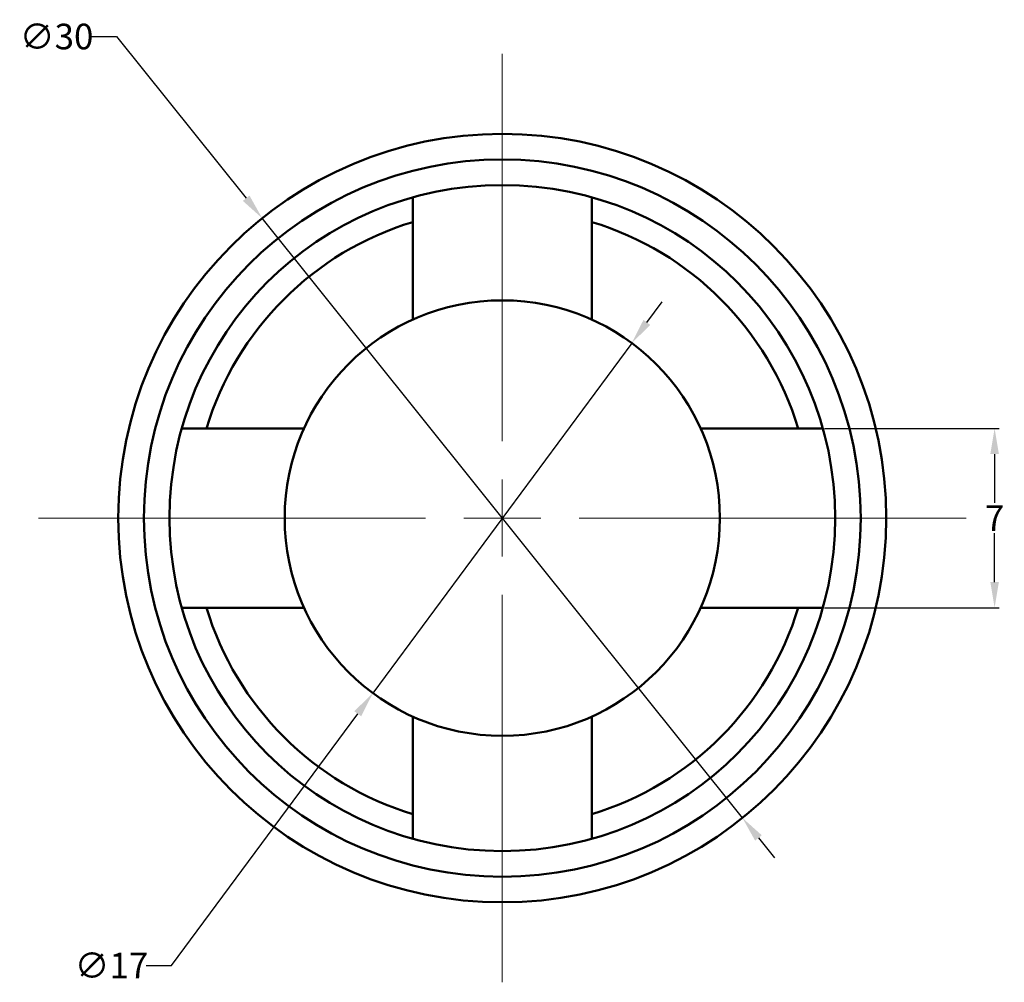
# Model space of a CAD drawing. Units: millimetres. Extents: x 31 to 232, y 35 to 192.
# Tile 4 of 5: x 43 to 82, y 154 to 192. Entities that reach past the tile are written whole.
import ezdxf

# ---------------------------------------------------------------- set-up
doc = ezdxf.new("R2010")
doc.units = ezdxf.units.MM
doc.header["$MEASUREMENT"] = 0
doc.linetypes.add('CENTER', pattern=[50.8, 31.75, -6.35, 6.35, -6.35])
for name, color, linetype, lineweight in [('M-CNTR', 1, 'CENTER', 18), ('M-DIMS', 2, 'Continuous', 25), ('M-OUTL', 7, 'Continuous', 50)]:
    doc.layers.add(name, color=color, linetype=linetype, lineweight=lineweight)
doc.styles.get("Standard").update_dxf_attribs({"font": 'arial.ttf'})
doc.dimstyles.get("Standard").update_dxf_attribs({"dimtxt": 1, "dimasz": 1, "dimexe": 0.18, "dimexo": 0.0625, "dimgap": 0.09, "dimtad": 0, "dimtih": 1, "dimtoh": 1, "dimdec": 0, "dimzin": 0, "dimdsep": 46, "dimtxsty": 'Standard', "dimcen": 0.09, "dimadec": 0, "dimazin": 0, "dimtfac": 1, "dimtdec": 0, "dimtofl": 0, "dimtmove": 0, "dimatfit": 3, "dimfxl": 1, "dimtolj": 1, "dimtzin": 0, "dimarcsym": 0})

# ---------------------------------------------------------------- blocks, each defined once
blk = doc.blocks.new('*U32')
at = {"layer": 'M-CNTR', "color": 0, "transparency": 16777216}
for p, q in [((0, 3), (0, 18.12)), ((-18.12, 0), (-3, 0)), ((3, 0), (18.12, 0)), ((0, -18.12), (0, -3))]:
    blk.add_line(p, q, dxfattribs=at)
at = {"layer": 'M-CNTR', "color": 0, "linetype": 'Continuous', "transparency": 16777216}
for p, q in [((0, -1.5), (0, 1.5)), ((-1.5, 0), (1.5, 0))]:
    blk.add_line(p, q, dxfattribs=at)
blk = doc.blocks.new('*D39')
at = {"layer": 'Defpoints', "color": 0, "transparency": 16777216}
for p in [(74.596, 175.753), (74.596, 168.753), (81.307, 168.753)]:
    blk.add_point(p, dxfattribs=at)
at = {"layer": 'M-DIMS', "color": 0, "lineweight": -2, "transparency": 16777216}
for p, q in [((74.659, 175.753), (81.487, 175.753)), ((81.307, 174.753), (81.307, 172.843)), ((81.307, 169.753), (81.307, 171.663)), ((74.659, 168.753), (81.487, 168.753))]:
    blk.add_line(p, q, dxfattribs=at)
at = {"layer": 'M-DIMS', "color": 0, "transparency": 16777216}
for points in [[(81.14, 174.753), (81.474, 174.753), (81.307, 175.753)], [(81.14, 169.753), (81.474, 169.753), (81.307, 168.753)]]:
    blk.add_solid(points, dxfattribs=at)
at = {"layer": 'M-DIMS', "color": 0, "transparency": 16777216, "insert": (81.307, 172.253), "char_height": 1, "attachment_point": 5}
blk.add_mtext('\\A1;7', dxfattribs=at)
blk = doc.blocks.new('*D40')
at = {"layer": 'Defpoints', "color": 0, "transparency": 16777216}
for p in [(52.696, 183.959), (71.456, 160.548)]:
    blk.add_point(p, dxfattribs=at)
at = {"layer": 'M-DIMS', "color": 0, "lineweight": -2, "transparency": 16777216}
for p, q in [((46.011, 191.053), (47.011, 191.053)), ((47.011, 191.053), (52.071, 184.739)), ((71.456, 160.548), (52.696, 183.959)), ((72.081, 159.767), (72.707, 158.987))]:
    blk.add_line(p, q, dxfattribs=at)
at = {"layer": 'M-DIMS', "color": 0, "transparency": 16777216}
for points in [[(52.201, 184.843), (51.941, 184.635), (52.696, 183.959)], [(72.211, 159.872), (71.951, 159.663), (71.456, 160.548)]]:
    blk.add_solid(points, dxfattribs=at)
at = {"layer": 'M-DIMS', "color": 0, "transparency": 16777216, "insert": (44.663, 191.053), "char_height": 1, "attachment_point": 5}
blk.add_mtext('\\A1;∅30', dxfattribs=at)
blk = doc.blocks.new('*D41')
at = {"layer": 'Defpoints', "color": 0, "transparency": 16777216}
for p in [(67.131, 179.087), (57.021, 165.419)]:
    blk.add_point(p, dxfattribs=at)
at = {"layer": 'M-DIMS', "color": 0, "lineweight": -2, "transparency": 16777216}
for p, q in [((67.725, 179.891), (68.32, 180.695)), ((67.131, 179.087), (57.021, 165.419)), ((49.158, 154.788), (56.427, 164.616)), ((48.158, 154.788), (49.158, 154.788))]:
    blk.add_line(p, q, dxfattribs=at)
blk.add_arc((62.076, 172.253), 8.5, 232.2984, 16.4262, dxfattribs=at)
at = {"layer": 'M-DIMS', "color": 0, "transparency": 16777216}
for points in [[(67.591, 179.99), (67.859, 179.792), (67.131, 179.087)], [(56.293, 164.715), (56.561, 164.516), (57.021, 165.419)]]:
    blk.add_solid(points, dxfattribs=at)
at = {"layer": 'M-DIMS', "color": 0, "transparency": 16777216, "insert": (46.807, 154.788), "char_height": 1, "attachment_point": 5}
blk.add_mtext('\\A1;∅17', dxfattribs=at)

msp = doc.modelspace()

# ---------------------------------------------------------------- linework, layer by layer
at = {"layer": 'M-OUTL'}
for p, q in [((58.576, 179.9993), (58.576, 184.7733)), ((65.576, 179.9993), (65.576, 184.7733)), ((49.556, 175.7533), (54.3301, 175.7533)), ((69.822, 175.7533), (74.596, 175.7533)), ((49.556, 168.7533), (54.3301, 168.7533)), ((69.822, 168.7533), (74.596, 168.7533)), ((58.576, 164.5073), (58.576, 159.7333)), ((65.576, 164.5073), (65.576, 159.7333))]:
    msp.add_line(p, q, dxfattribs=at)
for radius in [15, 14, 13, 8.5]:
    msp.add_circle((62.076, 172.2533), radius, dxfattribs=at)
for start, end in [(106.84753, 163.15247), (16.84753, 73.15247), (196.84753, 253.15247), (286.84753, 343.15247)]:
    msp.add_arc((62.076, 172.2533), 12.0762, start, end, dxfattribs=at)

# ---------------------------------------------------------------- block references
at = {"layer": 'M-CNTR'}
msp.add_blockref('*U32', (62.076, 172.2533), dxfattribs=at)

# ---------------------------------------------------------------- dimensions: what is measured, and where the dimension line sits
at = {"layer": 'M-DIMS'}
for p1, p2, picture, middle in [((71.4559, 160.5479), (52.6961, 183.9588), '*D40', (44.6629, 191.0529)), ((67.1306, 179.0871), (57.0214, 165.4195), '*D41', (46.8073, 154.7875))]:
    dim = msp.add_diameter_dim_2p(p1=p1, p2=p2, dimstyle='Standard', override={"dimclrd": 0, "dimclre": 0, "dimclrt": 0, "dimtofl": 1}, dxfattribs=at)
    dim.commit()
    dim.dimension.update_dxf_attribs({"geometry": picture, "text_midpoint": middle, "dimtype": 163})
dim = msp.add_linear_dim(base=(81.3072, 168.7533), p1=(74.596, 175.7533), p2=(74.596, 168.7533), angle=90, dimstyle='Standard', override={"dimclrd": 0, "dimclre": 0, "dimclrt": 0}, dxfattribs=at)
dim.commit()
dim.dimension.update_dxf_attribs({"geometry": '*D39', "text_midpoint": (81.3072, 172.2533)})

doc.saveas('drawing.dxf')
